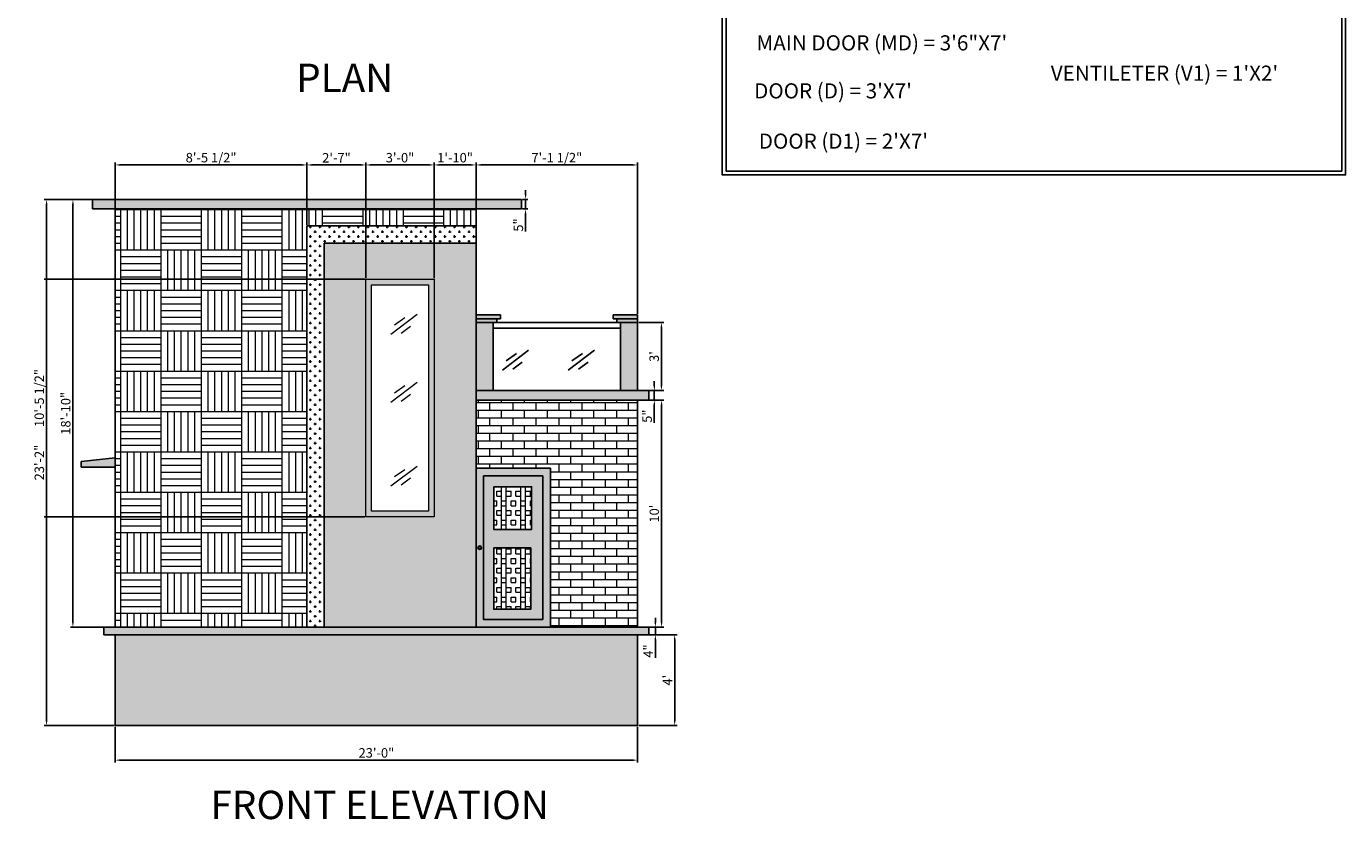
# Model space of a CAD drawing. Units: inches. Extents: x 1662 to 23131, y 1265 to 19127.
# Tile 6 of 26: x 12446 to 13143, y 5451 to 5870. Entities that reach past the tile are written whole.
import ezdxf

# ---------------------------------------------------------------- set-up
doc = ezdxf.new("R2010")
doc.units = ezdxf.units.IN
for name, color, linetype, lineweight in [('A-ANNO-DIMS', 4, 'Continuous', 18), ('A-ANNO-TEXT', 7, 'Continuous', 18), ('A-ANNO-TITL', 7, 'Continuous', 35), ('A-ANNO-TTLB', 7, 'Continuous', 25), ('A-ELEV', 7, 'Continuous', 25), ('A-ELEV-GLAZ', 4, 'Continuous', 18), ('A-ELEV-PATT', 8, 'Continuous', 13), ('A-ELEV-SURF-PATT', 252, 'Continuous', 13)]:
    doc.layers.add(name, color=color, linetype=linetype, lineweight=lineweight)
doc.styles.get("Standard").update_dxf_attribs({"font": 'arial.ttf'})
doc.dimstyles.new('ISO-25', dxfattribs={"dimtxt": 5, "dimasz": 2.5, "dimexe": 1.25, "dimexo": 0.625, "dimtad": 1, "dimlunit": 3, "dimtxsty": 'Standard', "dimcen": 2.5, "dimadec": 0, "dimazin": 0, "dimtfac": 1, "dimtmove": 0, "dimatfit": 3, "dimfxl": 1, "dimarcsym": 0})

# ---------------------------------------------------------------- blocks, each defined once
blk = doc.blocks.new('*D56')
at = {"layer": 'A-ANNO-DIMS', "color": 0, "lineweight": -2, "transparency": 16777216}
for p, q in [((12769.95, 5548.57), (12790.16, 5548.57)), ((12788.91, 5546.07), (12788.91, 5503.07)), ((12769.95, 5500.57), (12790.16, 5500.57))]:
    blk.add_line(p, q, dxfattribs=at)
at = {"layer": 'A-ANNO-DIMS', "color": 0, "transparency": 16777216}
for points in [[(12788.49, 5546.07), (12789.33, 5546.07), (12788.91, 5548.57)], [(12788.49, 5503.07), (12789.33, 5503.07), (12788.91, 5500.57)]]:
    blk.add_solid(points, dxfattribs=at)
at = {"layer": 'Defpoints', "color": 0, "transparency": 16777216}
for p in [(12769.33, 5548.57), (12769.33, 5500.57), (12788.91, 5500.57)]:
    blk.add_point(p, dxfattribs=at)
at = {"layer": 'A-ANNO-DIMS', "color": 0, "transparency": 16777216, "insert": (12785.78, 5524.57), "char_height": 5, "attachment_point": 5, "rotation": 90}
blk.add_mtext("4'", dxfattribs=at)
blk = doc.blocks.new('*D57')
at = {"layer": 'A-ANNO-DIMS', "color": 0, "lineweight": -2, "transparency": 16777216}
for p, q in [((12778.69, 5555.07), (12778.69, 5557.57)), ((12775.95, 5552.57), (12779.94, 5552.57)), ((12775.95, 5548.57), (12779.94, 5548.57)), ((12778.69, 5552.57), (12778.69, 5548.57)), ((12778.69, 5546.07), (12778.69, 5536.37))]:
    blk.add_line(p, q, dxfattribs=at)
at = {"layer": 'A-ANNO-DIMS', "color": 0, "transparency": 16777216}
for points in [[(12778.27, 5555.07), (12779.11, 5555.07), (12778.69, 5552.57)], [(12778.27, 5546.07), (12779.11, 5546.07), (12778.69, 5548.57)]]:
    blk.add_solid(points, dxfattribs=at)
at = {"layer": 'Defpoints', "color": 0, "transparency": 16777216}
for p in [(12775.33, 5552.57), (12775.33, 5548.57), (12778.69, 5548.57)]:
    blk.add_point(p, dxfattribs=at)
at = {"layer": 'A-ANNO-DIMS', "color": 0, "transparency": 16777216, "insert": (12775.56, 5539.97), "char_height": 5, "attachment_point": 5, "rotation": 90}
blk.add_mtext('4"', dxfattribs=at)
blk = doc.blocks.new('*D58')
at = {"layer": 'A-ANNO-DIMS', "color": 0, "lineweight": -2, "transparency": 16777216}
for p, q in [((12769.95, 5672.57), (12783.23, 5672.57)), ((12781.98, 5670.07), (12781.98, 5555.07)), ((12769.95, 5552.57), (12783.23, 5552.57))]:
    blk.add_line(p, q, dxfattribs=at)
at = {"layer": 'A-ANNO-DIMS', "color": 0, "transparency": 16777216}
for points in [[(12781.56, 5670.07), (12782.4, 5670.07), (12781.98, 5672.57)], [(12781.56, 5555.07), (12782.4, 5555.07), (12781.98, 5552.57)]]:
    blk.add_solid(points, dxfattribs=at)
at = {"layer": 'Defpoints', "color": 0, "transparency": 16777216}
for p in [(12769.33, 5672.57), (12769.33, 5552.57), (12781.98, 5552.57)]:
    blk.add_point(p, dxfattribs=at)
at = {"layer": 'A-ANNO-DIMS', "color": 0, "transparency": 16777216, "insert": (12778.8, 5612.57), "char_height": 5, "attachment_point": 5, "rotation": 90}
blk.add_mtext("10'", dxfattribs=at)
blk = doc.blocks.new('*D59')
at = {"layer": 'A-ANNO-DIMS', "color": 0, "lineweight": -2, "transparency": 16777216}
for p, q in [((12778.15, 5680.07), (12778.15, 5682.57)), ((12775.95, 5677.57), (12779.4, 5677.57)), ((12778.15, 5677.57), (12778.15, 5672.57)), ((12775.95, 5672.57), (12779.4, 5672.57)), ((12778.15, 5670.07), (12778.15, 5660.57))]:
    blk.add_line(p, q, dxfattribs=at)
at = {"layer": 'A-ANNO-DIMS', "color": 0, "transparency": 16777216}
for points in [[(12777.73, 5680.07), (12778.57, 5680.07), (12778.15, 5677.57)], [(12777.73, 5670.07), (12778.57, 5670.07), (12778.15, 5672.57)]]:
    blk.add_solid(points, dxfattribs=at)
at = {"layer": 'Defpoints', "color": 0, "transparency": 16777216}
for p in [(12775.33, 5677.57), (12775.33, 5672.57), (12778.15, 5672.57)]:
    blk.add_point(p, dxfattribs=at)
at = {"layer": 'A-ANNO-DIMS', "color": 0, "transparency": 16777216, "insert": (12774.98, 5664.07), "char_height": 5, "attachment_point": 5, "rotation": 90}
blk.add_mtext('5"', dxfattribs=at)
blk = doc.blocks.new('*D60')
at = {"layer": 'A-ANNO-DIMS', "color": 0, "lineweight": -2, "transparency": 16777216}
for p, q in [((12769.95, 5713.57), (12783.14, 5713.57)), ((12781.89, 5711.07), (12781.89, 5680.07)), ((12769.95, 5677.57), (12783.14, 5677.57))]:
    blk.add_line(p, q, dxfattribs=at)
at = {"layer": 'A-ANNO-DIMS', "color": 0, "transparency": 16777216}
for points in [[(12781.48, 5711.07), (12782.31, 5711.07), (12781.89, 5713.57)], [(12781.48, 5680.07), (12782.31, 5680.07), (12781.89, 5677.57)]]:
    blk.add_solid(points, dxfattribs=at)
at = {"layer": 'Defpoints', "color": 0, "transparency": 16777216}
for p in [(12769.33, 5713.57), (12769.33, 5677.57), (12781.89, 5677.57)]:
    blk.add_point(p, dxfattribs=at)
at = {"layer": 'A-ANNO-DIMS', "color": 0, "transparency": 16777216, "insert": (12778.71, 5695.57), "char_height": 5, "attachment_point": 5, "rotation": 90}
blk.add_mtext("3'", dxfattribs=at)
blk = doc.blocks.new('*D61')
at = {"layer": 'A-ANNO-DIMS', "color": 0, "lineweight": -2, "transparency": 16777216}
for p, q in [((12492.7, 5778.57), (12469.76, 5778.57)), ((12471.01, 5776.07), (12471.01, 5555.07)), ((12492.7, 5552.57), (12469.76, 5552.57))]:
    blk.add_line(p, q, dxfattribs=at)
at = {"layer": 'A-ANNO-DIMS', "color": 0, "transparency": 16777216}
for points in [[(12470.59, 5776.07), (12471.42, 5776.07), (12471.01, 5778.57)], [(12470.59, 5555.07), (12471.42, 5555.07), (12471.01, 5552.57)]]:
    blk.add_solid(points, dxfattribs=at)
at = {"layer": 'Defpoints', "color": 0, "transparency": 16777216}
for p in [(12493.33, 5778.57), (12471.01, 5552.57), (12493.33, 5552.57)]:
    blk.add_point(p, dxfattribs=at)
at = {"layer": 'A-ANNO-DIMS', "color": 0, "transparency": 16777216, "insert": (12467.83, 5665.57), "char_height": 5, "attachment_point": 5, "rotation": 90}
blk.add_mtext('18\'-10"', dxfattribs=at)
blk = doc.blocks.new('*D62')
at = {"layer": 'A-ANNO-DIMS', "color": 0, "lineweight": -2, "transparency": 16777216}
for p, q in [((12708.58, 5778.57), (12711.37, 5778.57)), ((12710.12, 5781.07), (12710.12, 5783.57)), ((12710.12, 5778.57), (12710.12, 5773.57)), ((12708.58, 5773.57), (12711.37, 5773.57)), ((12710.12, 5771.07), (12710.12, 5761.57))]:
    blk.add_line(p, q, dxfattribs=at)
at = {"layer": 'A-ANNO-DIMS', "color": 0, "transparency": 16777216}
for points in [[(12709.71, 5781.07), (12710.54, 5781.07), (12710.12, 5778.57)], [(12709.71, 5771.07), (12710.54, 5771.07), (12710.12, 5773.57)]]:
    blk.add_solid(points, dxfattribs=at)
at = {"layer": 'Defpoints', "color": 0, "transparency": 16777216}
for p in [(12707.96, 5778.57), (12707.96, 5773.57), (12710.12, 5773.57)]:
    blk.add_point(p, dxfattribs=at)
at = {"layer": 'A-ANNO-DIMS', "color": 0, "transparency": 16777216, "insert": (12706.96, 5765.07), "char_height": 5, "attachment_point": 5, "rotation": 90}
blk.add_mtext('5"', dxfattribs=at)
blk = doc.blocks.new('*D220')
at = {"layer": 'A-ANNO-DIMS', "color": 0, "lineweight": -2, "transparency": 16777216}
for p, q in [((12493.33, 5499.95), (12493.33, 5481.07)), ((12769.33, 5499.95), (12769.33, 5481.07)), ((12495.83, 5482.32), (12766.83, 5482.32))]:
    blk.add_line(p, q, dxfattribs=at)
at = {"layer": 'A-ANNO-DIMS', "color": 0, "transparency": 16777216}
for points in [[(12495.83, 5482.74), (12495.83, 5481.9), (12493.33, 5482.32)], [(12766.83, 5482.74), (12766.83, 5481.9), (12769.33, 5482.32)]]:
    blk.add_solid(points, dxfattribs=at)
at = {"layer": 'Defpoints', "color": 0, "transparency": 16777216}
for p in [(12493.33, 5500.57), (12769.33, 5500.57), (12769.33, 5482.32)]:
    blk.add_point(p, dxfattribs=at)
at = {"layer": 'A-ANNO-DIMS', "color": 0, "transparency": 16777216, "insert": (12631.33, 5485.5), "char_height": 5, "attachment_point": 5}
blk.add_mtext('23\'-0"', dxfattribs=at)
blk = doc.blocks.new('*D221')
at = {"layer": 'A-ANNO-DIMS', "color": 0, "lineweight": -2, "transparency": 16777216}
for p, q in [((12480.7, 5778.57), (12455.83, 5778.57)), ((12457.08, 5503.07), (12457.08, 5776.07)), ((12492.7, 5500.57), (12455.83, 5500.57))]:
    blk.add_line(p, q, dxfattribs=at)
at = {"layer": 'A-ANNO-DIMS', "color": 0, "transparency": 16777216}
for points in [[(12456.66, 5776.07), (12457.5, 5776.07), (12457.08, 5778.57)], [(12456.66, 5503.07), (12457.5, 5503.07), (12457.08, 5500.57)]]:
    blk.add_solid(points, dxfattribs=at)
at = {"layer": 'Defpoints', "color": 0, "transparency": 16777216}
for p in [(12457.08, 5778.57), (12481.33, 5778.57), (12493.33, 5500.57)]:
    blk.add_point(p, dxfattribs=at)
at = {"layer": 'A-ANNO-DIMS', "color": 0, "transparency": 16777216, "insert": (12453.9, 5639.57), "char_height": 5, "attachment_point": 5, "rotation": 90}
blk.add_mtext('23\'-2"', dxfattribs=at)
blk = doc.blocks.new('*D222')
at = {"layer": 'A-ANNO-DIMS', "color": 0, "lineweight": -2, "transparency": 16777216}
for p, q in [((12493.33, 5774.2), (12493.33, 5798.07)), ((12495.83, 5796.82), (12592.14, 5796.82)), ((12594.64, 5765.2), (12594.64, 5798.07))]:
    blk.add_line(p, q, dxfattribs=at)
at = {"layer": 'A-ANNO-DIMS', "color": 0, "transparency": 16777216}
for points in [[(12495.83, 5797.24), (12495.83, 5796.4), (12493.33, 5796.82)], [(12592.14, 5797.24), (12592.14, 5796.4), (12594.64, 5796.82)]]:
    blk.add_solid(points, dxfattribs=at)
at = {"layer": 'Defpoints', "color": 0, "transparency": 16777216}
for p in [(12594.64, 5796.82), (12493.33, 5773.57), (12594.64, 5764.57)]:
    blk.add_point(p, dxfattribs=at)
at = {"layer": 'A-ANNO-DIMS', "color": 0, "transparency": 16777216, "insert": (12543.99, 5800.03), "char_height": 5, "attachment_point": 5}
blk.add_mtext('8\'-5 1/2"', dxfattribs=at)
blk = doc.blocks.new('*D223')
at = {"layer": 'A-ANNO-DIMS', "color": 0, "lineweight": -2, "transparency": 16777216}
for p, q in [((12594.64, 5765.2), (12594.64, 5798.07)), ((12597.14, 5796.82), (12623.29, 5796.82)), ((12625.79, 5737.07), (12625.79, 5798.07))]:
    blk.add_line(p, q, dxfattribs=at)
at = {"layer": 'A-ANNO-DIMS', "color": 0, "transparency": 16777216}
for points in [[(12597.14, 5797.24), (12597.14, 5796.4), (12594.64, 5796.82)], [(12623.29, 5797.24), (12623.29, 5796.4), (12625.79, 5796.82)]]:
    blk.add_solid(points, dxfattribs=at)
at = {"layer": 'Defpoints', "color": 0, "transparency": 16777216}
for p in [(12625.79, 5796.82), (12594.64, 5764.57), (12625.79, 5736.45)]:
    blk.add_point(p, dxfattribs=at)
at = {"layer": 'A-ANNO-DIMS', "color": 0, "transparency": 16777216, "insert": (12610.22, 5799.96), "char_height": 5, "attachment_point": 5}
blk.add_mtext('2\'-7"', dxfattribs=at)
blk = doc.blocks.new('*D224')
at = {"layer": 'A-ANNO-DIMS', "color": 0, "lineweight": -2, "transparency": 16777216}
for p, q in [((12625.79, 5737.07), (12625.79, 5798.07)), ((12628.29, 5796.82), (12659.32, 5796.82)), ((12661.82, 5737.07), (12661.82, 5798.07))]:
    blk.add_line(p, q, dxfattribs=at)
at = {"layer": 'A-ANNO-DIMS', "color": 0, "transparency": 16777216}
for points in [[(12628.29, 5797.24), (12628.29, 5796.4), (12625.79, 5796.82)], [(12659.32, 5797.24), (12659.32, 5796.4), (12661.82, 5796.82)]]:
    blk.add_solid(points, dxfattribs=at)
at = {"layer": 'Defpoints', "color": 0, "transparency": 16777216}
for p in [(12661.82, 5796.82), (12625.79, 5736.45), (12661.82, 5736.45)]:
    blk.add_point(p, dxfattribs=at)
at = {"layer": 'A-ANNO-DIMS', "color": 0, "transparency": 16777216, "insert": (12643.8, 5800), "char_height": 5, "attachment_point": 5}
blk.add_mtext('3\'-0"', dxfattribs=at)
blk = doc.blocks.new('*D225')
at = {"layer": 'A-ANNO-DIMS', "color": 0, "lineweight": -2, "transparency": 16777216}
for p, q in [((12661.82, 5737.07), (12661.82, 5798.07)), ((12664.32, 5796.82), (12681.46, 5796.82)), ((12683.96, 5774.2), (12683.96, 5798.07))]:
    blk.add_line(p, q, dxfattribs=at)
at = {"layer": 'A-ANNO-DIMS', "color": 0, "transparency": 16777216}
for points in [[(12664.32, 5797.24), (12664.32, 5796.4), (12661.82, 5796.82)], [(12681.46, 5797.24), (12681.46, 5796.4), (12683.96, 5796.82)]]:
    blk.add_solid(points, dxfattribs=at)
at = {"layer": 'Defpoints', "color": 0, "transparency": 16777216}
for p in [(12683.96, 5796.82), (12683.96, 5773.57), (12661.82, 5736.45)]:
    blk.add_point(p, dxfattribs=at)
at = {"layer": 'A-ANNO-DIMS', "color": 0, "transparency": 16777216, "insert": (12672.89, 5800), "char_height": 5, "attachment_point": 5}
blk.add_mtext('1\'-10"', dxfattribs=at)
blk = doc.blocks.new('*D226')
at = {"layer": 'A-ANNO-DIMS', "color": 0, "lineweight": -2, "transparency": 16777216}
for p, q in [((12683.96, 5718.2), (12683.96, 5798.07)), ((12686.46, 5796.82), (12766.83, 5796.82)), ((12769.33, 5718.2), (12769.33, 5798.07))]:
    blk.add_line(p, q, dxfattribs=at)
at = {"layer": 'A-ANNO-DIMS', "color": 0, "transparency": 16777216}
for points in [[(12686.46, 5797.24), (12686.46, 5796.4), (12683.96, 5796.82)], [(12766.83, 5797.24), (12766.83, 5796.4), (12769.33, 5796.82)]]:
    blk.add_solid(points, dxfattribs=at)
at = {"layer": 'Defpoints', "color": 0, "transparency": 16777216}
for p in [(12769.33, 5796.82), (12683.96, 5717.57), (12769.33, 5717.57)]:
    blk.add_point(p, dxfattribs=at)
at = {"layer": 'A-ANNO-DIMS', "color": 0, "transparency": 16777216, "insert": (12726.64, 5800.03), "char_height": 5, "attachment_point": 5}
blk.add_mtext('7\'-1 1/2"', dxfattribs=at)
blk = doc.blocks.new('*D227')
at = {"layer": 'A-ANNO-DIMS', "color": 0, "lineweight": -2, "transparency": 16777216}
for p, q in [((12625.16, 5736.45), (12455.83, 5736.45)), ((12457.08, 5613.4), (12457.08, 5733.95)), ((12625.16, 5610.9), (12455.83, 5610.9))]:
    blk.add_line(p, q, dxfattribs=at)
at = {"layer": 'A-ANNO-DIMS', "color": 0, "transparency": 16777216}
for points in [[(12456.66, 5733.95), (12457.5, 5733.95), (12457.08, 5736.45)], [(12456.66, 5613.4), (12457.5, 5613.4), (12457.08, 5610.9)]]:
    blk.add_solid(points, dxfattribs=at)
at = {"layer": 'Defpoints', "color": 0, "transparency": 16777216}
for p in [(12457.08, 5736.45), (12625.79, 5736.45), (12625.79, 5610.9)]:
    blk.add_point(p, dxfattribs=at)
at = {"layer": 'A-ANNO-DIMS', "color": 0, "transparency": 16777216, "insert": (12453.87, 5673.67), "char_height": 5, "attachment_point": 5, "rotation": 90}
blk.add_mtext('10\'-5 1/2"', dxfattribs=at)

msp = doc.modelspace()

# ---------------------------------------------------------------- hatches: boundary and pattern name
at = {"layer": 'A-ELEV-PATT'}
h = msp.add_hatch(dxfattribs=at)
h.set_pattern_fill('AR-PARQ1', color=256, scale=0.07)
h.set_pattern_definition([(90, (-1841.556, 33.85), (-21.336, 21.336), [21.336, -21.336]), (90, (-1838, 33.85), (-21.336, 21.336), [21.336, -21.336]), (90, (-1834.444, 33.85), (-21.336, 21.336), [21.336, -21.336]), (90, (-1830.888, 33.85), (-21.336, 21.336), [21.336, -21.336]), (90, (-1827.332, 33.85), (-21.336, 21.336), [21.336, -21.336]), (90, (-1823.776, 33.85), (-21.336, 21.336), [21.336, -21.336]), (90, (-1820.22, 33.85), (-21.336, 21.336), [21.336, -21.336]), (0, (-1841.556, 55.186), (21.336, -21.336), [21.336, -21.336]), (0, (-1841.556, 58.742), (21.336, -21.336), [21.336, -21.336]), (0, (-1841.556, 62.298), (21.336, -21.336), [21.336, -21.336]), (0, (-1841.556, 65.854), (21.336, -21.336), [21.336, -21.336]), (0, (-1841.556, 69.41), (21.336, -21.336), [21.336, -21.336]), (0, (-1841.556, 72.966), (21.336, -21.336), [21.336, -21.336]), (0, (-1841.556, 76.522), (21.336, -21.336), [21.336, -21.336])])
h.paths.add_polyline_path([(12493.33, 5552.571), (12594.645, 5552.571), (12594.645, 5764.571), (12683.96, 5764.571), (12683.96, 5773.571), (12493.33, 5773.571)])
h = msp.add_hatch(dxfattribs=at)
h.set_pattern_fill('CROSS', color=256, scale=0.4)
h.set_pattern_definition([(0, (-1841.556, 33.8498), (2.54, 2.54), [1.27, -3.81]), (90, (-1840.921, 33.2148), (-2.54, 2.54), [1.27, -3.81])])
h.paths.add_polyline_path([(12603.645, 5755.571), (12683.96, 5755.571), (12683.96, 5764.571), (12594.645, 5764.571), (12594.645, 5552.571), (12603.645, 5552.571)])
h = msp.add_hatch(dxfattribs=at)
h.set_pattern_fill('AR-BRSTD', color=256, scale=0.06)
h.set_pattern_definition([(0, (-1841.556, 33.8498), (0, 4.064508), []), (90, (-1841.556, 33.85), (-6.096, 4.064508), [4.064508, -4.064508])])
h.paths.add_polyline_path([(12723.33, 5636.571), (12723.33, 5552.571), (12769.33, 5552.571), (12769.33, 5672.571), (12683.96, 5672.571), (12683.96, 5636.571)])
h = msp.add_hatch(dxfattribs=at)
h.set_pattern_fill('BOX', color=256, scale=0.4)
h.set_pattern_definition([(90, (-1841.556, 33.85), (-10.16, 6e-16), []), (90, (-1839.016, 33.85), (-10.16, 6e-16), []), (0, (-1841.556, 33.85), (0, 10.16), [-2.54, 2.54]), (0, (-1841.556, 36.39), (0, 10.16), [-2.54, 2.54]), (0, (-1841.556, 38.93), (0, 10.16), [2.54, -2.54]), (0, (-1841.556, 41.47), (0, 10.16), [2.54, -2.54]), (90, (-1836.476, 33.85), (-10.16, 6e-16), [2.54, -2.54]), (90, (-1833.936, 33.85), (-10.16, 6e-16), [2.54, -2.54])])
h.paths.add_polyline_path([(12693.355, 5604.275), (12713.328, 5604.275), (12713.328, 5626.746), (12693.355, 5626.746)])
h.paths.add_polyline_path([(12693.355, 5562.084), (12712.869, 5562.084), (12712.869, 5594.415), (12693.355, 5594.415)])
at = {"layer": 'A-ELEV-SURF-PATT'}
h = msp.add_hatch(color=256, dxfattribs=at)
h.dxf.hatch_style = 1
h.paths.add_polyline_path([(12683.96, 5677.571), (12683.96, 5672.571), (12775.33, 5672.571), (12775.33, 5677.571)])
h.paths.add_polyline_path([(12481.33, 5778.571), (12481.33, 5773.571), (12707.96, 5773.571), (12707.96, 5778.571)])
h.paths.add_polyline_path([(12493.33, 5637.071), (12493.33, 5642.071), (12475.33, 5640.071), (12475.33, 5637.071)])
h.paths.add_polyline_path([(12487.33, 5552.571), (12487.33, 5548.571), (12775.33, 5548.571), (12775.33, 5552.571)])
h = msp.add_hatch(color=256, dxfattribs=at)
h.dxf.hatch_style = 1
h.paths.add_polyline_path([(12683.96, 5552.571), (12683.96, 5755.571), (12603.645, 5755.571), (12603.645, 5552.571)])
h.paths.add_polyline_path([(12625.788, 5610.897), (12625.788, 5736.446), (12661.816, 5736.446), (12661.816, 5610.897)], flags=16)
h.paths.add_polyline_path([(12628.788, 5613.897), (12628.788, 5733.446), (12658.816, 5733.446), (12658.816, 5613.897)], flags=0)
h = msp.add_hatch(color=256, dxfattribs=at)
h.dxf.hatch_style = 1
h.paths.add_polyline_path([(12625.788, 5610.897), (12661.816, 5610.897), (12661.816, 5736.446), (12625.788, 5736.446)])
h.paths.add_polyline_path([(12628.788, 5733.446), (12658.816, 5733.446), (12658.816, 5613.897), (12628.788, 5613.897)], flags=16)
h = msp.add_hatch(color=256, dxfattribs=at)
h.dxf.hatch_style = 1
h.paths.add_polyline_path([(12683.96, 5717.571), (12683.96, 5715.571), (12694.96, 5715.571), (12696.96, 5715.571), (12696.96, 5717.571)])
h.paths.add_polyline_path([(12756.33, 5717.571), (12756.33, 5715.571), (12758.33, 5715.571), (12769.33, 5715.571), (12769.33, 5717.571)])
h = msp.add_hatch(color=256, dxfattribs=at)
h.dxf.hatch_style = 1
h.paths.add_polyline_path([(12694.96, 5713.571), (12694.96, 5715.571), (12683.96, 5715.571), (12683.96, 5713.571)])
h.paths.add_polyline_path([(12758.33, 5715.571), (12758.33, 5713.571), (12760.33, 5713.571), (12769.33, 5713.571), (12769.33, 5715.571)])
h = msp.add_hatch(color=256, dxfattribs=at)
h.dxf.hatch_style = 1
h.paths.add_polyline_path([(12758.33, 5715.571), (12758.33, 5713.571), (12760.33, 5713.571), (12769.33, 5713.571), (12769.33, 5715.571)])
h.paths.add_polyline_path([(12683.96, 5715.571), (12683.96, 5713.571), (12694.96, 5713.571), (12694.96, 5715.571)])
h = msp.add_hatch(color=256, dxfattribs=at)
h.dxf.hatch_style = 1
h.paths.add_polyline_path([(12692.96, 5713.571), (12683.96, 5713.571), (12683.96, 5677.571), (12692.96, 5677.571)])
h.paths.add_polyline_path([(12769.33, 5713.571), (12760.33, 5713.571), (12760.33, 5677.571), (12769.33, 5677.571)])
h = msp.add_hatch(color=256, dxfattribs=at)
h.dxf.hatch_style = 1
h.paths.add_polyline_path([(12683.96, 5552.571), (12723.33, 5552.571), (12723.33, 5636.571), (12683.96, 5636.571)])
h.paths.add_polyline_path([(12687.96, 5632.571), (12719.33, 5632.571), (12719.33, 5556.571), (12687.96, 5556.571)], flags=16)
h.paths.add_polyline_path([(12693.355, 5594.415), (12712.869, 5594.415), (12712.869, 5562.084), (12693.355, 5562.084)], flags=0)
h.paths.add_polyline_path([(12684.986, 5594.571, -1), (12686.933, 5594.571, -1)], flags=16)
h.paths.add_polyline_path([(12685.245, 5594.571, -1), (12686.674, 5594.571, -1)], flags=0)
h.paths.add_polyline_path([(12693.355, 5604.275), (12693.355, 5626.746), (12713.328, 5626.746), (12713.328, 5604.275)], flags=0)
h = msp.add_hatch(color=256, dxfattribs=at)
h.dxf.hatch_style = 1
h.paths.add_polyline_path([(12687.96, 5556.571), (12719.33, 5556.571), (12719.33, 5632.571), (12687.96, 5632.571)])
h.paths.add_polyline_path([(12693.355, 5604.275), (12693.355, 5626.746), (12713.328, 5626.746), (12713.328, 5604.275)], flags=16)
h.paths.add_polyline_path([(12712.869, 5594.415), (12712.869, 5562.084), (12693.355, 5562.084), (12693.355, 5594.415)], flags=16)
h = msp.add_hatch(color=256, dxfattribs=at)
h.dxf.hatch_style = 1
h.paths.add_polyline_path([(12686.933, 5594.571, 1), (12684.986, 5594.571, 1)])
h.paths.add_polyline_path([(12686.674, 5594.571, 1), (12685.245, 5594.571, 1)], flags=16)
h = msp.add_hatch(color=256, dxfattribs=at)
h.dxf.hatch_style = 1
h.paths.add_polyline_path([(12769.33, 5500.571), (12769.33, 5548.571), (12493.33, 5548.571), (12493.33, 5500.571)])

# ---------------------------------------------------------------- linework, layer by layer
at = {"layer": 'A-ANNO-TTLB'}
for points in [[(12814.019, 5975.699), (13143.349, 5975.699), (13143.349, 5791.544), (12814.019, 5791.544)], [(12816.019, 5973.699), (13141.349, 5973.699), (13141.349, 5793.544), (12816.019, 5793.544)]]:
    msp.add_lwpolyline(points, close=True, dxfattribs=at)
at = {"layer": 'A-ELEV'}
for p, q in [((12481.33, 5778.571), (12707.96, 5778.571)), ((12481.33, 5773.571), (12481.33, 5778.571)), ((12707.96, 5778.571), (12707.96, 5773.571)), ((12481.33, 5773.571), (12707.96, 5773.571)), ((12493.33, 5773.571), (12493.33, 5552.571)), ((12683.96, 5773.571), (12683.96, 5552.571)), ((12594.645, 5764.571), (12594.645, 5552.571)), ((12594.645, 5764.571), (12683.96, 5764.571)), ((12603.645, 5755.571), (12603.645, 5552.571)), ((12603.645, 5755.571), (12683.96, 5755.571)), ((12696.96, 5717.571), (12683.96, 5717.571)), ((12694.96, 5715.571), (12683.96, 5715.571)), ((12694.96, 5713.571), (12694.96, 5715.571)), ((12694.96, 5715.571), (12696.96, 5715.571)), ((12696.96, 5715.571), (12696.96, 5717.571)), ((12756.33, 5715.571), (12756.33, 5717.571)), ((12756.33, 5717.571), (12769.33, 5717.571)), ((12758.33, 5715.571), (12756.33, 5715.571)), ((12758.33, 5713.571), (12758.33, 5715.571)), ((12758.33, 5715.571), (12769.33, 5715.571)), ((12769.33, 5717.571), (12769.33, 5715.571)), ((12769.33, 5715.571), (12769.33, 5713.571)), ((12683.96, 5713.571), (12769.33, 5713.571)), ((12692.96, 5713.571), (12692.96, 5677.571)), ((12692.96, 5713.571), (12694.96, 5713.571)), ((12692.96, 5710.571), (12760.33, 5710.571)), ((12760.33, 5713.571), (12758.33, 5713.571)), ((12760.33, 5713.571), (12760.33, 5677.571)), ((12769.33, 5713.571), (12769.33, 5677.571)), ((12697.856, 5688.418), (12711.752, 5698.96)), ((12699.857, 5693.338), (12705.369, 5697.192)), ((12732.645, 5688.418), (12746.541, 5698.96)), ((12734.646, 5693.338), (12740.158, 5697.192)), ((12703.385, 5688.934), (12708.345, 5692.677)), ((12738.174, 5688.934), (12743.134, 5692.677)), ((12683.96, 5677.571), (12775.33, 5677.571)), ((12775.33, 5672.571), (12775.33, 5677.571)), ((12683.96, 5672.571), (12775.33, 5672.571)), ((12769.33, 5672.571), (12769.33, 5552.571)), ((12493.33, 5642.071), (12475.33, 5640.071)), ((12475.33, 5637.071), (12475.33, 5640.071)), ((12493.33, 5637.071), (12493.33, 5642.071)), ((12493.33, 5637.071), (12475.33, 5637.071)), ((12683.96, 5636.571), (12723.33, 5636.571)), ((12687.96, 5632.571), (12719.33, 5632.571)), ((12687.96, 5632.571), (12687.96, 5556.571)), ((12719.33, 5632.571), (12719.33, 5556.571)), ((12723.33, 5636.571), (12723.33, 5552.571)), ((12687.96, 5556.571), (12719.33, 5556.571)), ((12487.33, 5552.571), (12775.33, 5552.571)), ((12487.33, 5548.571), (12487.33, 5552.571)), ((12487.33, 5548.571), (12775.33, 5548.571)), ((12493.33, 5548.571), (12493.33, 5500.571)), ((12769.33, 5548.571), (12769.33, 5500.571)), ((12775.33, 5548.571), (12775.33, 5552.571)), ((12493.33, 5500.571), (12769.33, 5500.571))]:
    msp.add_line(p, q, dxfattribs=at)
for points in [[(12693.355, 5626.746), (12713.328, 5626.746), (12713.328, 5604.275), (12693.355, 5604.275)], [(12693.355, 5594.415), (12712.869, 5594.415), (12712.869, 5562.084), (12693.355, 5562.084)]]:
    msp.add_lwpolyline(points, close=True, dxfattribs=at)
for radius in [0.974, 0.714]:
    msp.add_circle((12685.96, 5594.571), radius, dxfattribs=at)
at = {"layer": 'A-ELEV-GLAZ'}
for p, q in [((12638.892, 5707.353), (12652.789, 5717.895)), ((12640.894, 5712.273), (12646.405, 5716.126)), ((12644.421, 5707.868), (12649.382, 5711.612)), ((12638.892, 5671.508), (12652.789, 5682.05)), ((12640.894, 5676.428), (12646.405, 5680.281)), ((12644.421, 5672.023), (12649.382, 5675.767)), ((12638.892, 5627.189), (12652.789, 5637.731)), ((12640.894, 5632.109), (12646.405, 5635.963)), ((12644.421, 5627.705), (12649.382, 5631.448))]:
    msp.add_line(p, q, dxfattribs=at)
for points in [[(12625.788, 5736.446), (12661.816, 5736.446), (12661.816, 5610.897), (12625.788, 5610.897)], [(12628.788, 5733.446), (12658.816, 5733.446), (12658.816, 5613.897), (12628.788, 5613.897)]]:
    msp.add_lwpolyline(points, close=True, dxfattribs=at)

# ---------------------------------------------------------------- texts
at = {"layer": 'A-ANNO-TEXT', "char_height": 10, "attachment_point": 1}
for s, insert in [('{\\H0.8x;MAIN DOOR (MD) = 3\'6"X7\'}', (12832.104, 5865.322)), ("{\\H0.8x;VENTILETER (V1) = 1'X2'}", (12987.604, 5849.299)), ("{\\H0.8x;DOOR (D) = 3'X7'}", (12830.892, 5839.964)), ("{\\H0.8x; DOOR (D1) = 2'X7'}", (12830.892, 5813.388))]:
    msp.add_mtext_dynamic_manual_height_columns(s, width=1142.59551, gutter_width=12.5, heights=[0], dxfattribs=dict(at, insert=insert))
at = {"layer": 'A-ANNO-TITL', "char_height": 15, "attachment_point": 1}
for s, insert in [('PLAN', (12588.92, 5850.346)), ('FRONT ELEVATION', (12543.662, 5466.158))]:
    msp.add_mtext_dynamic_manual_height_columns(s, width=1142.59551, gutter_width=12.5, heights=[0], dxfattribs=dict(at, insert=insert))

# ---------------------------------------------------------------- dimensions: what is measured, and where the dimension line sits
at = {"layer": 'A-ANNO-DIMS'}
for base, p1, p2, picture, middle in [((12594.645, 5796.821), (12493.33, 5773.571), (12594.645, 5764.571), '*D222', (12543.987, 5800.031)), ((12769.33, 5796.821), (12683.96, 5717.571), (12769.33, 5717.571), '*D226', (12726.645, 5800.031)), ((12625.788, 5796.821), (12594.645, 5764.571), (12625.788, 5736.446), '*D223', (12610.216, 5799.956)), ((12661.816, 5796.821), (12625.788, 5736.446), (12661.816, 5736.446), '*D224', (12643.802, 5800.001)), ((12683.96, 5796.821), (12661.816, 5736.446), (12683.96, 5773.571), '*D225', (12672.888, 5799.999)), ((12769.33, 5482.321), (12493.33, 5500.571), (12769.33, 5500.571), '*D220', (12631.33, 5485.501))]:
    dim = msp.add_linear_dim(base=base, p1=p1, p2=p2, dimstyle='ISO-25', override={"dimdec": 1, "dimlfac": 1, "dimrnd": 0, "dimzin": 1, "dimdsep": 46, "dimlunit": 4, "dimfrac": 2}, dxfattribs=at)
    dim.commit()
    dim.dimension.update_dxf_attribs({"geometry": picture, "text_midpoint": middle})
for base, p1, p2, override, picture, middle in [((12457.08, 5778.571), (12493.33, 5500.571), (12481.33, 5778.571), {"dimdec": 1, "dimlfac": 1, "dimrnd": 0, "dimzin": 1, "dimdsep": 46, "dimlunit": 4, "dimfrac": 2}, '*D221', (12453.9, 5639.571)), ((12471.007, 5552.571), (12493.33, 5778.571), (12493.33, 5552.571), {"dimclrd": 0, "dimclre": 0, "dimclrt": 0}, '*D61', (12467.829, 5665.571)), ((12710.123, 5773.571), (12707.96, 5778.571), (12707.96, 5773.571), {"dimclrd": 0, "dimclre": 0, "dimclrt": 0}, '*D62', (12706.955, 5765.073)), ((12457.08, 5736.446), (12625.788, 5610.897), (12625.788, 5736.446), {"dimdec": 1, "dimlfac": 1, "dimrnd": 0, "dimzin": 1, "dimdsep": 46, "dimlunit": 4, "dimfrac": 2}, '*D227', (12453.869, 5673.672)), ((12781.893, 5677.571), (12769.33, 5713.571), (12769.33, 5677.571), {"dimclrd": 0, "dimclre": 0, "dimclrt": 0}, '*D60', (12778.714, 5695.571)), ((12778.15, 5672.571), (12775.33, 5677.571), (12775.33, 5672.571), {"dimclrd": 0, "dimclre": 0, "dimclrt": 0}, '*D59', (12774.982, 5664.073)), ((12781.98, 5552.571), (12769.33, 5672.571), (12769.33, 5552.571), {"dimclrd": 0, "dimclre": 0, "dimclrt": 0}, '*D58', (12778.803, 5612.571)), ((12778.689, 5548.571), (12775.33, 5552.571), (12775.33, 5548.571), {"dimclrd": 0, "dimclre": 0, "dimclrt": 0}, '*D57', (12775.564, 5539.972)), ((12788.908, 5500.571), (12769.33, 5548.571), (12769.33, 5500.571), {"dimclrd": 0, "dimclre": 0, "dimclrt": 0}, '*D56', (12785.783, 5524.571))]:
    dim = msp.add_linear_dim(base=base, p1=p1, p2=p2, angle=90, dimstyle='ISO-25', override=override, dxfattribs=at)
    dim.commit()
    dim.dimension.update_dxf_attribs({"geometry": picture, "text_midpoint": middle})

doc.saveas('drawing.dxf')
